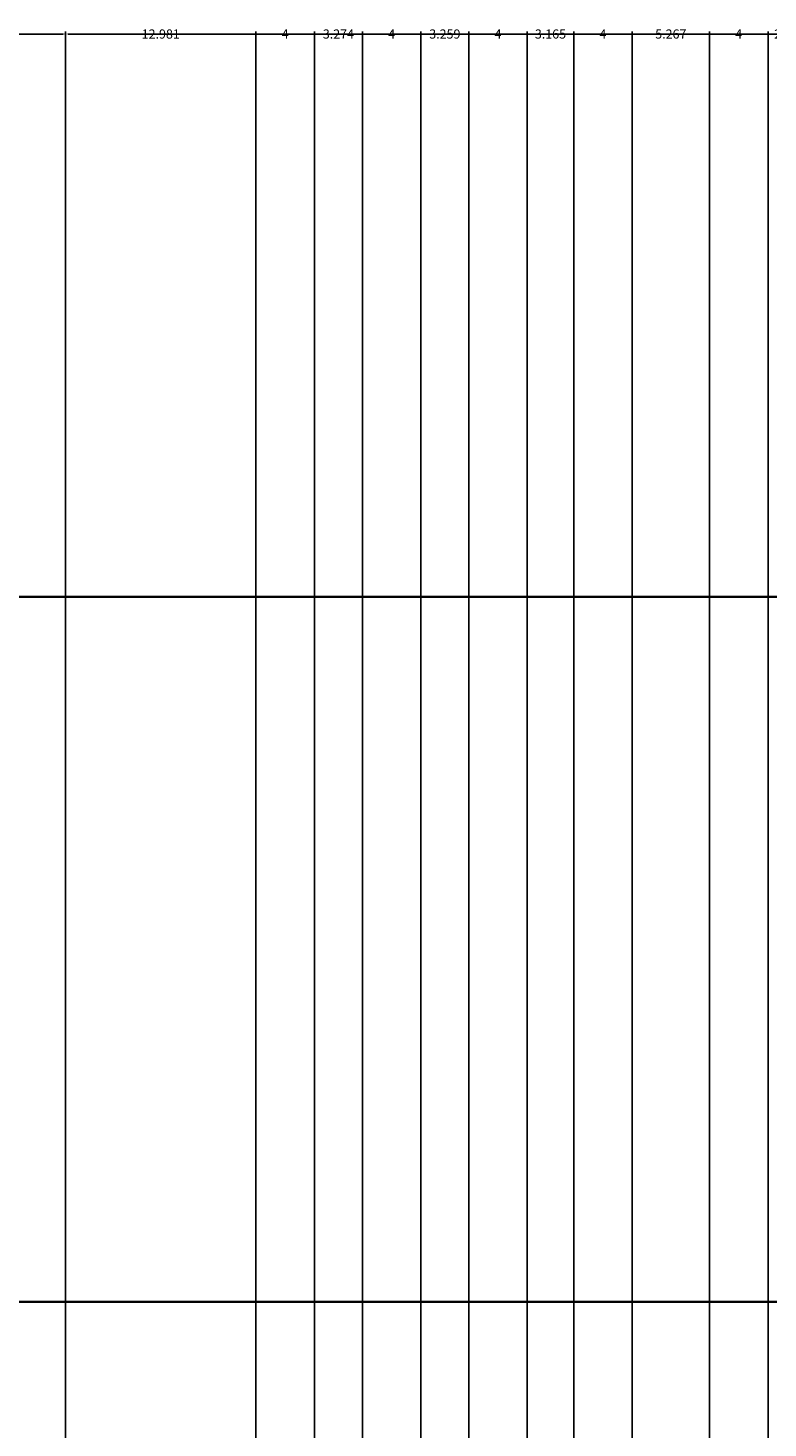
# Model space of a CAD drawing. Units: inches. Extents: x -13 to 809, y 112 to 656.
# Tile 36 of 55: x 339 to 389, y 561 to 656. Entities that reach past the tile are written whole.
import ezdxf

# ---------------------------------------------------------------- set-up
doc = ezdxf.new("R2010")
doc.units = ezdxf.units.IN
doc.header["$MEASUREMENT"] = 0
doc.layers.add('A-ANNO-DIMS', color=2, linetype='Continuous', lineweight=18)
doc.layers.add('A-ELEV', color=7, linetype='Continuous', lineweight=35)
doc.styles.get("Standard").update_dxf_attribs({"font": 'arial.ttf'})
doc.dimstyles.get("Standard").update_dxf_attribs({"dimtxt": 0.625, "dimasz": 0.18, "dimexe": 0.18, "dimexo": 0.0625, "dimgap": 0.09, "dimtad": 0, "dimtih": 1, "dimtoh": 1, "dimdec": 4, "dimzin": 0, "dimdsep": 46, "dimlunit": 4, "dimtxsty": 'Standard', "dimcen": 0.09, "dimadec": 0, "dimazin": 0, "dimtfac": 1, "dimtdec": 4, "dimtofl": 0, "dimtmove": 0, "dimatfit": 3, "dimfxl": 1, "dimtolj": 1, "dimtzin": 0, "dimarcsym": 0})

# ---------------------------------------------------------------- blocks, each defined once
blk = doc.blocks.new('*D25')
at = {"layer": 'A-ANNO-DIMS', "color": 0, "lineweight": -2, "transparency": 16777216}
for p, q in [((311.699, 617.433), (311.699, 655.963)), ((311.879, 655.783), (325.464, 655.783)), ((341.227, 655.783), (327.643, 655.783)), ((341.407, 524.343), (341.407, 655.963))]:
    blk.add_line(p, q, dxfattribs=at)
at = {"layer": 'A-ANNO-DIMS', "color": 0, "transparency": 16777216}
for points in [[(311.879, 655.813), (311.879, 655.753), (311.699, 655.783)], [(341.227, 655.813), (341.227, 655.753), (341.407, 655.783)]]:
    blk.add_solid(points, dxfattribs=at)
at = {"layer": 'Defpoints', "color": 0, "transparency": 16777216}
for p in [(341.407, 655.783), (311.699, 617.371), (341.407, 524.281)]:
    blk.add_point(p, dxfattribs=at)
at = {"layer": 'A-ANNO-DIMS', "color": 0, "transparency": 16777216, "insert": (326.553, 655.783), "char_height": 0.625, "attachment_point": 5}
blk.add_mtext('\\A1;29.71', dxfattribs=at)
blk = doc.blocks.new('*D26')
at = {"layer": 'A-ANNO-DIMS', "color": 0, "lineweight": -2, "transparency": 16777216}
for p, q in [((341.407, 524.343), (341.407, 655.963)), ((341.587, 655.783), (405.138, 655.783)), ((470.92, 655.783), (407.369, 655.783)), ((471.1, 470.939), (471.1, 655.963))]:
    blk.add_line(p, q, dxfattribs=at)
at = {"layer": 'A-ANNO-DIMS', "color": 0, "transparency": 16777216}
for points in [[(341.587, 655.813), (341.587, 655.753), (341.407, 655.783)], [(470.92, 655.813), (470.92, 655.753), (471.1, 655.783)]]:
    blk.add_solid(points, dxfattribs=at)
at = {"layer": 'Defpoints', "color": 0, "transparency": 16777216}
for p in [(471.1, 655.783), (341.407, 524.281), (471.1, 470.877)]:
    blk.add_point(p, dxfattribs=at)
at = {"layer": 'A-ANNO-DIMS', "color": 0, "transparency": 16777216, "insert": (406.253, 655.783), "char_height": 0.625, "attachment_point": 5}
blk.add_mtext('\\A1;129.7', dxfattribs=at)
blk = doc.blocks.new('*D53')
at = {"layer": 'A-ANNO-DIMS', "color": 0, "lineweight": -2, "transparency": 16777216}
for p, q in [((341.407, 524.343), (341.407, 655.963)), ((341.587, 655.783), (346.6, 655.783)), ((354.209, 655.783), (349.195, 655.783)), ((354.389, 524.343), (354.389, 655.963))]:
    blk.add_line(p, q, dxfattribs=at)
at = {"layer": 'A-ANNO-DIMS', "color": 0, "transparency": 16777216}
for points in [[(341.587, 655.813), (341.587, 655.753), (341.407, 655.783)], [(354.209, 655.813), (354.209, 655.753), (354.389, 655.783)]]:
    blk.add_solid(points, dxfattribs=at)
at = {"layer": 'Defpoints', "color": 0, "transparency": 16777216}
for p in [(354.389, 655.783), (341.407, 524.281), (354.389, 524.281)]:
    blk.add_point(p, dxfattribs=at)
at = {"layer": 'A-ANNO-DIMS', "color": 0, "transparency": 16777216, "insert": (347.898, 655.783), "char_height": 0.625, "attachment_point": 5}
blk.add_mtext('\\A1;12.981', dxfattribs=at)
blk = doc.blocks.new('*D54')
at = {"layer": 'A-ANNO-DIMS', "color": 0, "lineweight": -2, "transparency": 16777216}
for p, q in [((354.389, 524.343), (354.389, 655.963)), ((354.569, 655.783), (356.082, 655.783)), ((358.209, 655.783), (356.695, 655.783)), ((358.389, 524.343), (358.389, 655.963))]:
    blk.add_line(p, q, dxfattribs=at)
at = {"layer": 'A-ANNO-DIMS', "color": 0, "transparency": 16777216}
for points in [[(354.569, 655.813), (354.569, 655.753), (354.389, 655.783)], [(358.209, 655.813), (358.209, 655.753), (358.389, 655.783)]]:
    blk.add_solid(points, dxfattribs=at)
at = {"layer": 'Defpoints', "color": 0, "transparency": 16777216}
for p in [(358.389, 655.783), (354.389, 524.281), (358.389, 524.281)]:
    blk.add_point(p, dxfattribs=at)
at = {"layer": 'A-ANNO-DIMS', "color": 0, "transparency": 16777216, "insert": (356.389, 655.783), "char_height": 0.625, "attachment_point": 5}
blk.add_mtext('\\A1;4', dxfattribs=at)
blk = doc.blocks.new('*D55')
at = {"layer": 'A-ANNO-DIMS', "color": 0, "lineweight": -2, "transparency": 16777216}
for p, q in [((358.389, 524.343), (358.389, 655.963)), ((358.569, 655.783), (358.883, 655.783)), ((361.483, 655.783), (361.169, 655.783)), ((361.663, 524.343), (361.663, 655.963))]:
    blk.add_line(p, q, dxfattribs=at)
at = {"layer": 'A-ANNO-DIMS', "color": 0, "transparency": 16777216}
for points in [[(358.569, 655.813), (358.569, 655.753), (358.389, 655.783)], [(361.483, 655.813), (361.483, 655.753), (361.663, 655.783)]]:
    blk.add_solid(points, dxfattribs=at)
at = {"layer": 'Defpoints', "color": 0, "transparency": 16777216}
for p in [(361.663, 655.783), (358.389, 524.281), (361.663, 524.281)]:
    blk.add_point(p, dxfattribs=at)
at = {"layer": 'A-ANNO-DIMS', "color": 0, "transparency": 16777216, "insert": (360.026, 655.783), "char_height": 0.625, "attachment_point": 5}
blk.add_mtext('\\A1;3.274', dxfattribs=at)
blk = doc.blocks.new('*D56')
at = {"layer": 'A-ANNO-DIMS', "color": 0, "lineweight": -2, "transparency": 16777216}
for p, q in [((361.663, 524.343), (361.663, 655.963)), ((361.843, 655.783), (363.356, 655.783)), ((365.483, 655.783), (363.969, 655.783)), ((365.663, 524.343), (365.663, 655.963))]:
    blk.add_line(p, q, dxfattribs=at)
at = {"layer": 'A-ANNO-DIMS', "color": 0, "transparency": 16777216}
for points in [[(361.843, 655.813), (361.843, 655.753), (361.663, 655.783)], [(365.483, 655.813), (365.483, 655.753), (365.663, 655.783)]]:
    blk.add_solid(points, dxfattribs=at)
at = {"layer": 'Defpoints', "color": 0, "transparency": 16777216}
for p in [(365.663, 655.783), (361.663, 524.281), (365.663, 524.281)]:
    blk.add_point(p, dxfattribs=at)
at = {"layer": 'A-ANNO-DIMS', "color": 0, "transparency": 16777216, "insert": (363.663, 655.783), "char_height": 0.625, "attachment_point": 5}
blk.add_mtext('\\A1;4', dxfattribs=at)
blk = doc.blocks.new('*D57')
at = {"layer": 'A-ANNO-DIMS', "color": 0, "lineweight": -2, "transparency": 16777216}
for p, q in [((365.663, 524.343), (365.663, 655.963)), ((365.843, 655.783), (366.147, 655.783)), ((368.741, 655.783), (368.437, 655.783)), ((368.921, 524.343), (368.921, 655.963))]:
    blk.add_line(p, q, dxfattribs=at)
at = {"layer": 'A-ANNO-DIMS', "color": 0, "transparency": 16777216}
for points in [[(365.843, 655.813), (365.843, 655.753), (365.663, 655.783)], [(368.741, 655.813), (368.741, 655.753), (368.921, 655.783)]]:
    blk.add_solid(points, dxfattribs=at)
at = {"layer": 'Defpoints', "color": 0, "transparency": 16777216}
for p in [(368.921, 655.783), (365.663, 524.281), (368.921, 524.281)]:
    blk.add_point(p, dxfattribs=at)
at = {"layer": 'A-ANNO-DIMS', "color": 0, "transparency": 16777216, "insert": (367.292, 655.783), "char_height": 0.625, "attachment_point": 5}
blk.add_mtext('\\A1;3.259', dxfattribs=at)
blk = doc.blocks.new('*D58')
at = {"layer": 'A-ANNO-DIMS', "color": 0, "lineweight": -2, "transparency": 16777216}
for p, q in [((368.921, 524.343), (368.921, 655.963)), ((369.101, 655.783), (370.615, 655.783)), ((372.741, 655.783), (371.228, 655.783)), ((372.921, 524.343), (372.921, 655.963))]:
    blk.add_line(p, q, dxfattribs=at)
at = {"layer": 'A-ANNO-DIMS', "color": 0, "transparency": 16777216}
for points in [[(369.101, 655.813), (369.101, 655.753), (368.921, 655.783)], [(372.741, 655.813), (372.741, 655.753), (372.921, 655.783)]]:
    blk.add_solid(points, dxfattribs=at)
at = {"layer": 'Defpoints', "color": 0, "transparency": 16777216}
for p in [(372.921, 655.783), (368.921, 524.281), (372.921, 524.281)]:
    blk.add_point(p, dxfattribs=at)
at = {"layer": 'A-ANNO-DIMS', "color": 0, "transparency": 16777216, "insert": (370.921, 655.783), "char_height": 0.625, "attachment_point": 5}
blk.add_mtext('\\A1;4', dxfattribs=at)
blk = doc.blocks.new('*D59')
at = {"layer": 'A-ANNO-DIMS', "color": 0, "lineweight": -2, "transparency": 16777216}
for p, q in [((372.921, 524.343), (372.921, 655.963)), ((373.101, 655.783), (373.357, 655.783)), ((375.907, 655.783), (375.651, 655.783)), ((376.087, 524.343), (376.087, 655.963))]:
    blk.add_line(p, q, dxfattribs=at)
at = {"layer": 'A-ANNO-DIMS', "color": 0, "transparency": 16777216}
for points in [[(373.101, 655.813), (373.101, 655.753), (372.921, 655.783)], [(375.907, 655.813), (375.907, 655.753), (376.087, 655.783)]]:
    blk.add_solid(points, dxfattribs=at)
at = {"layer": 'Defpoints', "color": 0, "transparency": 16777216}
for p in [(376.087, 655.783), (372.921, 524.281), (376.087, 524.281)]:
    blk.add_point(p, dxfattribs=at)
at = {"layer": 'A-ANNO-DIMS', "color": 0, "transparency": 16777216, "insert": (374.504, 655.783), "char_height": 0.625, "attachment_point": 5}
blk.add_mtext('\\A1;3.165', dxfattribs=at)
blk = doc.blocks.new('*D60')
at = {"layer": 'A-ANNO-DIMS', "color": 0, "lineweight": -2, "transparency": 16777216}
for p, q in [((376.087, 524.343), (376.087, 655.963)), ((376.267, 655.783), (377.78, 655.783)), ((379.907, 655.783), (378.393, 655.783)), ((380.087, 524.343), (380.087, 655.963))]:
    blk.add_line(p, q, dxfattribs=at)
at = {"layer": 'A-ANNO-DIMS', "color": 0, "transparency": 16777216}
for points in [[(376.267, 655.813), (376.267, 655.753), (376.087, 655.783)], [(379.907, 655.813), (379.907, 655.753), (380.087, 655.783)]]:
    blk.add_solid(points, dxfattribs=at)
at = {"layer": 'Defpoints', "color": 0, "transparency": 16777216}
for p in [(380.087, 655.783), (376.087, 524.281), (380.087, 524.281)]:
    blk.add_point(p, dxfattribs=at)
at = {"layer": 'A-ANNO-DIMS', "color": 0, "transparency": 16777216, "insert": (378.087, 655.783), "char_height": 0.625, "attachment_point": 5}
blk.add_mtext('\\A1;4', dxfattribs=at)
blk = doc.blocks.new('*D61')
at = {"layer": 'A-ANNO-DIMS', "color": 0, "lineweight": -2, "transparency": 16777216}
for p, q in [((380.087, 524.343), (380.087, 655.963)), ((380.267, 655.783), (381.576, 655.783)), ((385.174, 655.783), (383.865, 655.783)), ((385.354, 524.343), (385.354, 655.963))]:
    blk.add_line(p, q, dxfattribs=at)
at = {"layer": 'A-ANNO-DIMS', "color": 0, "transparency": 16777216}
for points in [[(380.267, 655.813), (380.267, 655.753), (380.087, 655.783)], [(385.174, 655.813), (385.174, 655.753), (385.354, 655.783)]]:
    blk.add_solid(points, dxfattribs=at)
at = {"layer": 'Defpoints', "color": 0, "transparency": 16777216}
for p in [(385.354, 655.783), (380.087, 524.281), (385.354, 524.281)]:
    blk.add_point(p, dxfattribs=at)
at = {"layer": 'A-ANNO-DIMS', "color": 0, "transparency": 16777216, "insert": (382.72, 655.783), "char_height": 0.625, "attachment_point": 5}
blk.add_mtext('\\A1;5.267', dxfattribs=at)
blk = doc.blocks.new('*D62')
at = {"layer": 'A-ANNO-DIMS', "color": 0, "lineweight": -2, "transparency": 16777216}
for p, q in [((385.354, 524.343), (385.354, 655.963)), ((385.534, 655.783), (387.047, 655.783)), ((389.174, 655.783), (387.66, 655.783)), ((389.354, 524.343), (389.354, 655.963))]:
    blk.add_line(p, q, dxfattribs=at)
at = {"layer": 'A-ANNO-DIMS', "color": 0, "transparency": 16777216}
for points in [[(385.534, 655.813), (385.534, 655.753), (385.354, 655.783)], [(389.174, 655.813), (389.174, 655.753), (389.354, 655.783)]]:
    blk.add_solid(points, dxfattribs=at)
at = {"layer": 'Defpoints', "color": 0, "transparency": 16777216}
for p in [(389.354, 655.783), (385.354, 524.281), (389.354, 524.281)]:
    blk.add_point(p, dxfattribs=at)
at = {"layer": 'A-ANNO-DIMS', "color": 0, "transparency": 16777216, "insert": (387.354, 655.783), "char_height": 0.625, "attachment_point": 5}
blk.add_mtext('\\A1;4', dxfattribs=at)
blk = doc.blocks.new('*D63')
at = {"layer": 'A-ANNO-DIMS', "color": 0, "lineweight": -2, "transparency": 16777216}
for p, q in [((389.354, 524.343), (389.354, 655.963)), ((389.534, 655.783), (389.692, 655.783)), ((392.148, 655.783), (391.989, 655.783)), ((392.328, 524.343), (392.328, 655.963))]:
    blk.add_line(p, q, dxfattribs=at)
at = {"layer": 'A-ANNO-DIMS', "color": 0, "transparency": 16777216}
for points in [[(389.534, 655.813), (389.534, 655.753), (389.354, 655.783)], [(392.148, 655.813), (392.148, 655.753), (392.328, 655.783)]]:
    blk.add_solid(points, dxfattribs=at)
at = {"layer": 'Defpoints', "color": 0, "transparency": 16777216}
for p in [(392.328, 655.783), (389.354, 524.281), (392.328, 524.281)]:
    blk.add_point(p, dxfattribs=at)
at = {"layer": 'A-ANNO-DIMS', "color": 0, "transparency": 16777216, "insert": (390.841, 655.783), "char_height": 0.625, "attachment_point": 5}
blk.add_mtext('\\A1;2.974', dxfattribs=at)

msp = doc.modelspace()

# ---------------------------------------------------------------- linework, layer by layer
at = {"layer": 'A-ELEV'}
for p, q in [((311.6991, 617.3708), (621.008, 617.3708)), ((292.923, 569.2414), (644.6221, 569.2414))]:
    msp.add_line(p, q, dxfattribs=at)

# ---------------------------------------------------------------- dimensions: what is measured, and where the dimension line sits
at = {"layer": 'A-ANNO-DIMS'}
for base, p1, p2, override, picture, middle in [((341.4072, 655.7828), (311.6991, 617.3708), (341.4072, 524.281), {"dimdec": 2, "dimlfac": 1, "dimrnd": 0, "dimzin": 0, "dimdsep": 46, "dimlunit": 2}, '*D25', (326.5531, 655.7828)), ((471.0998, 655.7828), (341.4072, 524.281), (471.0998, 470.8765), {"dimdec": 1, "dimlfac": 1, "dimrnd": 0, "dimzin": 0, "dimdsep": 46, "dimlunit": 2}, '*D26', (406.2535, 655.7828)), ((354.3886, 655.7828), (341.4072, 524.281), (354.3886, 524.281), {"dimdec": 3, "dimlfac": 1, "dimrnd": 0, "dimzin": 0, "dimdsep": 46, "dimlunit": 2}, '*D53', (347.8979, 655.7828)), ((358.3886, 655.7828), (354.3886, 524.281), (358.3886, 524.281), {"dimdec": 0, "dimlfac": 1, "dimrnd": 0, "dimzin": 0, "dimdsep": 46, "dimlunit": 2}, '*D54', (356.3886, 655.7828)), ((361.6625, 655.7828), (358.3886, 524.281), (361.6625, 524.281), {"dimdec": 3, "dimlfac": 1, "dimrnd": 0, "dimzin": 0, "dimdsep": 46, "dimlunit": 2}, '*D55', (360.0256, 655.7828)), ((365.6625, 655.7828), (361.6625, 524.281), (365.6625, 524.281), {"dimdec": 0, "dimlfac": 1, "dimrnd": 0, "dimzin": 0, "dimdsep": 46, "dimlunit": 2}, '*D56', (363.6625, 655.7828)), ((368.9215, 655.7828), (365.6625, 524.281), (368.9215, 524.281), {"dimdec": 3, "dimlfac": 1, "dimrnd": 0, "dimzin": 0, "dimdsep": 46, "dimlunit": 2}, '*D57', (367.292, 655.7828)), ((372.9215, 655.7828), (368.9215, 524.281), (372.9215, 524.281), {"dimdec": 0, "dimlfac": 1, "dimrnd": 0, "dimzin": 0, "dimdsep": 46, "dimlunit": 2}, '*D58', (370.9215, 655.7828)), ((376.0866, 655.7828), (372.9215, 524.281), (376.0866, 524.281), {"dimdec": 3, "dimlfac": 1, "dimrnd": 0, "dimzin": 0, "dimdsep": 46, "dimlunit": 2}, '*D59', (374.504, 655.7828)), ((380.0866, 655.7828), (376.0866, 524.281), (380.0866, 524.281), {"dimdec": 0, "dimlfac": 1, "dimrnd": 0, "dimzin": 0, "dimdsep": 46, "dimlunit": 2}, '*D60', (378.0866, 655.7828)), ((385.3536, 655.7828), (380.0866, 524.281), (385.3536, 524.281), {"dimdec": 3, "dimlfac": 1, "dimrnd": 0, "dimzin": 0, "dimdsep": 46, "dimlunit": 2}, '*D61', (382.7201, 655.7828)), ((389.3536, 655.7828), (385.3536, 524.281), (389.3536, 524.281), {"dimdec": 0, "dimlfac": 1, "dimrnd": 0, "dimzin": 0, "dimdsep": 46, "dimlunit": 2}, '*D62', (387.3536, 655.7828)), ((392.3277, 655.7828), (389.3536, 524.281), (392.3277, 524.281), {"dimdec": 3, "dimlfac": 1, "dimrnd": 0, "dimzin": 0, "dimdsep": 46, "dimlunit": 2}, '*D63', (390.8407, 655.7828))]:
    dim = msp.add_linear_dim(base=base, p1=p1, p2=p2, dimstyle='Standard', override=override, dxfattribs=at)
    dim.commit()
    dim.dimension.update_dxf_attribs({"geometry": picture, "text_midpoint": middle})

doc.saveas('drawing.dxf')
